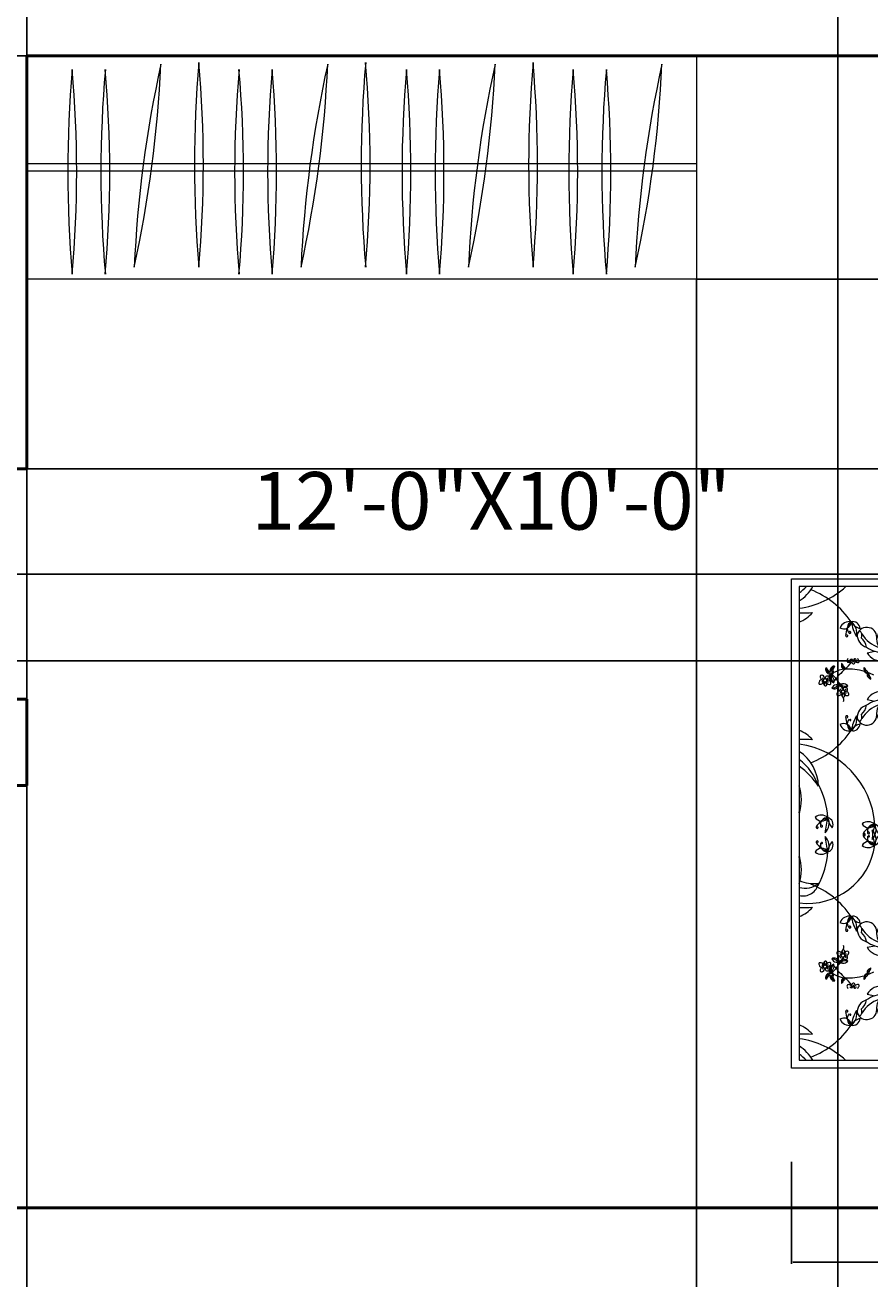
# Model space of a CAD drawing. Units: inches. Extents: x 3 to 576, y -689 to 51.
# Tile 5 of 21: x 111 to 199, y -514 to -383. Entities that reach past the tile are written whole.
import ezdxf

# ---------------------------------------------------------------- set-up
doc = ezdxf.new("R2010")
doc.units = ezdxf.units.IN
doc.header["$MEASUREMENT"] = 0
for name, color, linetype, lineweight in [('A-ANNO-DIMS', 2, 'Continuous', 18), ('A-AREA-IDEN', 7, 'Continuous', 18), ('A-FURN', 8, 'Continuous', 18), ('A-WALL', 7, 'Continuous', 50)]:
    doc.layers.add(name, color=color, linetype=linetype, lineweight=lineweight)
doc.styles.get("Standard").update_dxf_attribs({"font": 'arial.ttf'})
doc.dimstyles.get("Standard").update_dxf_attribs({"dimtxt": 0.18, "dimasz": 0.18, "dimexe": 0.18, "dimexo": 0.0625, "dimgap": 0.09, "dimtad": 0, "dimtih": 1, "dimtoh": 1, "dimdec": 0, "dimzin": 0, "dimdsep": 46, "dimlunit": 3, "dimtxsty": 'Standard', "dimcen": 0.09, "dimadec": 0, "dimazin": 0, "dimtfac": 1, "dimtdec": 0, "dimtofl": 0, "dimtmove": 0, "dimatfit": 3, "dimfxl": 1, "dimtolj": 1, "dimtzin": 0, "dimarcsym": 0})

# ---------------------------------------------------------------- blocks, each defined once
blk = doc.blocks.new('BED-DOUBLE')
for p, q in [((59.45, 69.91), (59.45, 0)), ((53.63, 58.35), (53.63, 67.49)), ((49.06, 62.92), (58.2, 62.92)), ((0, 60.68), (25.18, 60.68)), ((0, 9.72), (0, 60.68)), ((25.18, 60.68), (25.18, 56.73)), ((0.81, 59.87), (0.81, 10.53)), ((24.37, 59.87), (0.81, 59.87)), ((24.37, 56.73), (24.37, 59.87)), ((19.95, 13.6), (19.95, 56.73)), ((20.82, 13.66), (20.82, 56.73)), ((38.97, 55.99), (39.54, 56.55)), ((39.54, 56.55), (42.51, 54.01)), ((39.25, 53.16), (38.97, 55.99)), ((59.45, 55.93), (40.27, 55.93)), ((48.41, 55.93), (48.41, 13.98)), ((58.56, 13.98), (58.56, 55.93)), ((42.51, 54.01), (44.49, 51.31)), ((7.9, 52.98), (8.69, 53.14)), ((38.97, 49.62), (39.25, 53.16)), ((44.49, 51.31), (46.33, 46.22)), ((13.08, 20.76), (13.08, 49.15)), ((38.55, 46.5), (38.97, 49.62)), ((7.9, 48.1), (8.69, 47.94)), ((37.7, 44.66), (38.55, 46.5)), ((46.33, 46.22), (48.41, 38.59)), ((37.13, 42.39), (37.7, 44.66)), ((38.97, 42.11), (37.13, 42.39)), ((43.07, 40.55), (38.97, 42.11)), ((41.87, 14.23), (41.76, 41.05)), ((42.58, 14.23), (42.48, 40.78)), ((48.41, 36.72), (43.07, 40.55)), ((44.78, 14.2), (44.43, 39.58)), ((45.5, 14.17), (45.15, 39.06)), ((7.9, 22.3), (8.69, 22.46)), ((7.9, 17.41), (8.69, 17.26)), ((24.37, 10.53), (24.37, 13.61)), ((25.18, 13.59), (25.18, 9.72)), ((0.81, 10.53), (24.37, 10.53)), ((53.63, 11.56), (53.63, 2.42)), ((25.18, 9.72), (0, 9.72)), ((49.06, 6.99), (58.2, 6.99))]:
    blk.add_line(p, q)
for points in [[(47.8, 55.93), (47.8, 69.91), (59.45, 69.91)], [(53.63, 62.92), (52.22, 62.1)], [(53.63, 62.92), (55.04, 62.1)], [(59.45, 13.98), (47.8, 13.98), (47.8, 0), (59.45, 0)], [(53.63, 6.99), (52.22, 7.81)], [(53.63, 6.99), (55.04, 7.81)]]:
    blk.add_lwpolyline(points)
for points in [[(33.13, 56.7, 0.001242), (19.87, 56.73, -0.127202), (13.26, 58.14)], [(57.71, 51.91, 0.074897), (53.14, 51.83, -0.472817)], [(52.89, 35.28, 0.14099), (57.55, 35.14, 0.235245)], [(52.89, 32.3, -0.14099), (57.55, 32.44, -0.235245)], [(57.71, 18, -0.074897), (53.14, 18.08, 0.472817)], [(21.37, 13.68, 0.056112), (17.53, 13.18, 0.095341), (13.82, 12.19)]]:
    blk.add_lwpolyline(points, format="xyb")
for centre, radius in [((53.63, 62.92), 3.26), ((53.63, 62.92), 1.63), ((3.49, 50.11), 0.178), ((5.36, 48.94), 0.178), ((5.36, 21.45), 0.178), ((3.49, 20.29), 0.178), ((53.63, 6.99), 3.26), ((53.63, 6.99), 1.63)]:
    blk.add_circle(centre, radius)
for centre, radius, start, end in [((-2.47, 63.69), 5.54, 306.3036, 316.4814), ((-1.64, 62.09), 4.45, 303.4617, 330.1116), ((-0.42, 66.67), 9.13, 277.745, 311.8856), ((-1.32, 51.05), 9.13, 34.3865, 68.5908), ((13.3, 57.49), 0.645, 93.98, 207.3412), ((-0.61, 59.6), 3.71, 292.5547, 318.9546), ((1.38, 69.77), 12.63, 267.4081, 273.6519), ((6, 55.22), 1.01, 77.7115, 159.0387), ((5.45, 56.23), 0.762, 238.4633, 358.2869), ((7.95, 54.69), 2.31, 138.8402, 177.9352), ((6.56, 55.55), 0.747, 117.6827, 223.7762), ((6.39, 55.47), 0.757, 2.9516, 103.728), ((12.45, 57.59), 6.39, 192.5173, 207.1824), ((5.37, 55.04), 1.44, 345.4653, 54.2343), ((7.54, 57.02), 1.56, 211.3827, 255.2969), ((-59.69, 49.98), 72.78, 359.3433, 5.6887), ((37.8, 120.65), 64.12, 265.8294, 271.553), ((64.29, 55.36), 26.39, 177.4519, 191.3392), ((6.09, 55.1), 0.0988, 223.7762, 159.7183), ((7.84, 54.58), 1.05, 350.264, 160.8688), ((8.16, 54.83), 1.31, 175.969, 254.3045), ((6.7, 54.8), 0.643, 333.9755, 53.2681), ((10.15, 56.66), 3.3, 211.2614, 251.7045), ((10.53, 54.2), 1.67, 84.9449, 172.8857), ((11.17, 53.54), 1.62, 111.5819, 201.4221), ((10.7, 54.68), 1.18, 354.4856, 91.0538), ((8.16, 57.76), 5.29, 303.6671, 333.2997), ((5.76, 54.77), 0.113, 177.9352, 11.4834), ((5.81, 54.78), 0.0551, 11.4834, 127.9409), ((6.41, 53.42), 1.4, 6.1662, 51.5825), ((9.88, 56.69), 3.75, 236.2883, 266.5076), ((10.9, 54.49), 2.03, 182.3591, 234.0401), ((9.83, 55.04), 2.1, 265.2933, 346.921), ((6.09, 52.15), 0.294, 127.7621, 169.0403), ((5.94, 52.4), 0.414, 265.053, 338.3618), ((6.48, 51.84), 0.541, 113.4276, 137.6104), ((6.42, 52.4), 0.178, 183.2768, 356.7232), ((6.55, 52.07), 0.291, 139.7889, 227.6792), ((6.25, 52.01), 0.368, 350.3487, 43.6538), ((6.93, 52.39), 0.428, 198.7263, 262.5032), ((6.59, 52.19), 0.17, 1.1081, 91.8675), ((6.7, 52.15), 0.297, 11.5637, 52.6358), ((9.4, 53.85), 1.74, 209.9085, 343.1337), ((10.13, 52.75), 0.434, 167.3041, 285.1471), ((11.31, 50.67), 2.7, 122.7011, 126.3445), ((11.81, 53.58), 2.23, 199.2822, 299.1751), ((10.62, 50.95), 1.43, 41.5653, 105.1471), ((12.57, 55.82), 2.9, 238.8218, 279.1554), ((11.31, 50.67), 2.7, 55.785, 94.7304), ((12.31, 52.24), 0.842, 30.0293, 52.325), ((3.75, 51.26), 0.199, 124.3538, 214.3923), ((4.04, 51.23), 0.464, 190.3057, 287.1958), ((4.17, 51.39), 0.538, 176.9701, 248.2913), ((8.01, 54.23), 5.2, 212.6784, 216.3746), ((3.99, 51.27), 0.206, 216.3746, 291.7548), ((4.48, 51.12), 0.464, 122.8155, 187.3992), ((4.12, 50.93), 0.155, 289.3605, 111.7548), ((4.24, 50.93), 0.155, 221.8703, 44.2646), ((4.69, 51.06), 0.538, 109.4799, 177.6828), ((4.4, 51.4), 0.199, 56.8636, 146.9021), ((4.5, 51.18), 0.206, 148.8844, 224.2646), ((8.78, 48.6), 5.2, 145.1882, 148.8844), ((5.81, 48.38), 2.9, 94.756, 119.2041), ((11.99, 44.2), 9.55, 132.2412, 142.1744), ((7.17, 51.8), 1.97, 178.3264, 187.1302), ((5.04, 51.53), 0.367, 11.3256, 64.4621), ((6.29, 52.06), 1.1, 190.2588, 210.656), ((5.55, 51.61), 0.336, 188.3432, 274.2869), ((5.84, 51.79), 0.586, 210.656, 242.6341), ((6.28, 52.3), 1.12, 218.2101, 226.3071), ((5.45, 51.35), 0.142, 325.7657, 67.4417), ((1.03, 56.11), 6.64, 313.1541, 322.0459), ((5.96, 45.49), 5.79, 73.5842, 93.8277), ((5.91, 52.13), 0.137, 142.4737, 265.053), ((6.46, 51.97), 0.153, 227.6792, 350.3487), ((5.87, 52.08), 0.583, 353.0852, 15.7171), ((6.91, 52.1), 0.138, 255.2356, 54.9248), ((9.52, 51.39), 1.97, 178.3264, 187.1302), ((7.39, 51.11), 0.367, 11.3256, 64.4621), ((8.64, 51.64), 1.1, 190.2588, 210.656), ((7.9, 51.19), 0.336, 188.3432, 274.2869), ((8.19, 51.38), 0.586, 210.656, 242.6341), ((8.64, 51.88), 1.12, 218.2101, 226.3071), ((7.81, 50.93), 0.142, 325.7657, 67.4417), ((11.41, 53.92), 2.01, 277.436, 299.9149), ((12.48, 52.59), 1.05, 221.5653, 293.8354), ((12.31, 52.24), 0.842, 314.4517, 333.558), ((58.53, 49.42), 9.37, 165.1039, 191.0369), ((51.31, 43.01), 9.01, 65.1316, 101.7583), ((723.03, 13.38), 666.43, 176.68521, 177.14978), ((2.98, 49.84), 0.137, 142.4737, 265.053), ((3.16, 49.87), 0.294, 61.2196, 169.0403), ((3, 50.12), 0.414, 265.053, 338.3618), ((3.35, 50.47), 0.351, 157.4086, 261.4386), ((3.15, 50.48), 0.176, 58.0499, 135.6268), ((3.55, 49.55), 0.541, 113.4276, 137.6104), ((3.34, 50.37), 0.118, 172.906, 277.132), ((2.95, 50.16), 0.561, 14.7558, 58.0499), ((3.62, 49.79), 0.291, 139.7889, 227.6792), ((3.53, 49.68), 0.153, 227.6792, 350.3487), ((3.74, 50.31), 0.243, 36.1046, 181.4281), ((2.93, 49.79), 0.583, 353.0852, 15.7171), ((3.31, 49.72), 0.368, 350.3487, 43.6538), ((3.59, 50.5), 0.245, 270.0645, 331.1507), ((3.8, 50.44), 0.28, 221.8413, 265.7877), ((4, 50.1), 0.428, 198.7263, 262.5032), ((3.66, 49.9), 0.17, 1.1081, 91.8675), ((3.8, 50.33), 0.174, 263.7526, 41.7054), ((3.76, 49.86), 0.297, 11.5637, 86.365), ((5.81, 48.38), 2.9, 124.0033, 132.4917), ((3.98, 49.81), 0.138, 255.2356, 54.9248), ((2.83, 48.01), 3.1, 63.7819, 68.2913), ((4.48, 50.4), 0.493, 128.3208, 208.8162), ((4.57, 50.43), 0.59, 207.7043, 254.3516), ((4.94, 50.48), 0.812, 157.2305, 229.0635), ((4.67, 50.75), 0.478, 174.4544, 220.6188), ((4.19, 50.1), 0.812, 270.278, 342.111), ((4.73, 49.08), 0.574, 98.7227, 159.3375), ((1.96, 48.08), 3.48, 30.544, 49.818), ((3.87, 50.06), 0.574, 340.0041, 40.6188), ((4.57, 50.12), 0.478, 278.7227, 324.8872), ((4.49, 49.73), 0.493, 290.5253, 358.5375), ((5.45, 49.87), 0.493, 182.8499, 266.1226), ((5.26, 50.22), 0.478, 231.7607, 277.9252), ((5.63, 50.31), 0.812, 214.5369, 286.3699), ((5.4, 49.18), 0.574, 37.3105, 97.9252), ((8.21, 50.67), 0.336, 147.5332, 233.4768), ((7.94, 50.71), 0.142, 354.3784, 96.0543), ((8.51, 50.85), 0.586, 179.1859, 211.164), ((5.96, 45.49), 5.79, 63.0032, 69.8941), ((8.95, 51.12), 1.1, 211.164, 231.5612), ((9.15, 52.01), 1.97, 234.6898, 243.4936), ((9.16, 51), 1.12, 195.5129, 203.6099), ((7.9, 50.27), 0.367, 357.3579, 50.4944), ((9.48, 50.34), 0.135, 12.7051, 190.4384), ((9.56, 50.36), 0.219, 190.4384, 10.4136), ((11.81, 47.5), 2.23, 60.8249, 160.7178), ((32.84, 49.05), 5.69, 336.2616, 11.3392), ((4.44, 49.82), 0.59, 244.9899, 291.6373), ((4.85, 48.67), 0.137, 142.4737, 265.053), ((5.03, 48.7), 0.294, 61.2196, 169.0403), ((4.88, 48.95), 0.414, 265.053, 338.3618), ((5.23, 49.31), 0.351, 157.4086, 261.4386), ((5.03, 49.32), 0.176, 58.0499, 135.6268), ((5.43, 48.38), 0.541, 113.4276, 137.6104), ((5.21, 49.21), 0.118, 172.906, 277.132), ((4.83, 48.99), 0.561, 14.7558, 58.0499), ((1.96, 48.08), 3.48, 23.0501, 23.8477), ((5.5, 48.62), 0.291, 139.7889, 227.6792), ((5.4, 48.52), 0.153, 227.6792, 350.3487), ((5.61, 49.14), 0.243, 36.1046, 181.4281), ((4.81, 48.63), 0.583, 353.0852, 15.7171), ((5.47, 49.97), 0.59, 265.0106, 311.658), ((1.96, 48.08), 3.48, 357.1071, 4.7585), ((5.19, 48.56), 0.368, 350.3487, 43.6538), ((5.47, 49.33), 0.245, 270.0645, 331.1507), ((5.68, 49.27), 0.28, 221.8413, 265.7877), ((5.87, 48.94), 0.428, 198.7263, 262.5032), ((5.53, 48.74), 0.17, 1.1081, 91.8675), ((5.68, 49.17), 0.174, 263.7526, 41.7054), ((5.64, 48.7), 0.297, 11.5637, 86.365), ((5.85, 48.65), 0.138, 255.2356, 54.9248), ((9.4, 47.23), 1.74, 16.8663, 150.0915), ((10.13, 48.33), 0.434, 74.8529, 192.6959), ((10.62, 50.13), 1.43, 254.8529, 318.4347), ((11.41, 47.16), 2.01, 60.0851, 82.564), ((12.48, 48.49), 1.05, 66.1646, 138.4347), ((12.31, 48.84), 0.842, 307.675, 336.7144), ((12.31, 48.84), 0.842, 23.229, 45.5483), ((8.16, 46.25), 1.31, 105.6955, 184.031), ((6.41, 47.66), 1.4, 308.4175, 353.8338), ((10.15, 44.42), 3.3, 108.2955, 148.7386), ((9.88, 44.39), 3.75, 93.4924, 123.7117), ((10.9, 46.59), 2.03, 125.9599, 177.6409), ((11.17, 47.54), 1.62, 158.5779, 248.4181), ((9.83, 46.04), 2.1, 13.079, 94.7067), ((11.31, 50.41), 2.7, 233.6555, 237.2989), ((12.57, 45.26), 2.9, 79.7133, 121.1782), ((11.31, 50.41), 2.7, 265.2696, 304.215), ((8.16, 43.32), 5.29, 21.4941, 56.3329), ((65.19, 44.49), 16.25, 168.0397, 199.2615), ((5.76, 46.31), 0.113, 348.5166, 182.0648), ((7.95, 46.39), 2.31, 182.0648, 221.1598), ((5.81, 46.3), 0.0551, 232.0591, 348.5166), ((6.56, 45.54), 0.747, 136.2238, 242.3173), ((6.13, 45.97), 0.0595, 200.2667, 136.2271), ((5.37, 46.05), 1.44, 305.7657, 14.5347), ((12.45, 43.49), 6.39, 152.8176, 167.4827), ((7.84, 46.5), 1.05, 199.1312, 9.736), ((6.7, 46.28), 0.643, 306.7319, 26.0245), ((10.53, 46.88), 1.67, 187.1143, 275.0551), ((10.7, 46.4), 1.18, 268.9462, 5.5144), ((63.55, 37.54), 27.11, 160.1194, 169.3383), ((32.41, 42.33), 25.35, 352.2196, 9.497), ((-0.61, 41.48), 3.71, 41.0454, 67.4453), ((-1.32, 50.03), 9.13, 291.4092, 325.6135), ((5.45, 44.85), 0.762, 1.7131, 121.5367), ((6, 45.86), 1.01, 200.9613, 282.2885), ((6.39, 45.61), 0.757, 256.272, 357.0484), ((7.54, 44.06), 1.56, 104.7031, 148.6173), ((1.38, 31.32), 12.63, 86.3481, 92.5919), ((-0.42, 34.41), 9.13, 4.4623, 82.255), ((-1.64, 38.99), 4.45, 1.272, 56.5383), ((-2.47, 37.39), 5.54, 17.8504, 53.6964), ((37.07, 42.55), 0.169, 178.8623, 289.7536), ((-4.03, 34.48), 8.25, 34.0123, 54.053), ((-5.31, 35.11), 9.13, 4.4623, 27.4146), ((61.64, 37.91), 12.33, 169.8617, 193.6238), ((45.23, 36.98), 12.46, 351.5249, 13.96), ((-3.99, 37.66), 5.02, 343.5431, 17.0202), ((-6.58, 35.67), 7.42, 4.3787, 5.6357), ((-11.66, 31.77), 13.27, 19.7217, 19.9028), ((3.11, 35.07), 1.01, 47.7873, 129.1145), ((3.14, 36.22), 0.762, 208.5391, 328.3627), ((4.54, 33.64), 2.31, 108.9159, 148.011), ((3.76, 35.07), 0.747, 87.7585, 193.852), ((9.89, 33.91), 6.39, 162.593, 177.2582), ((2.48, 35.23), 1.44, 315.5411, 24.3101), ((5.35, 35.86), 1.56, 181.4585, 225.3727), ((3.58, 35.09), 0.757, 333.0274, 73.8037), ((8, 34.37), 1.01, 47.7873, 129.1145), ((50.55, 43.52), 8.57, 264.0129, 285.8293), ((2.68, 34.8), 0.113, 148.011, 341.5592), ((2.73, 34.78), 0.0551, 341.5592, 98.0167), ((3.13, 34.92), 0.0988, 193.852, 129.9245), ((8.03, 35.52), 0.762, 208.5391, 328.3627), ((7.57, 34.1), 0.113, 148.011, 341.5592), ((7.57, 33.97), 0.113, 18.4408, 211.989), ((9.43, 32.94), 2.31, 108.9159, 148.011), ((7.62, 34.08), 0.0551, 341.5592, 98.0167), ((7.62, 33.99), 0.0551, 261.9833, 18.4408), ((8.65, 34.38), 0.747, 87.7585, 193.852), ((8.02, 34.22), 0.0988, 193.852, 129.9245), ((7.37, 34.53), 1.44, 315.5411, 24.3101), ((14.78, 33.21), 6.39, 162.593, 177.2582), ((7.37, 33.54), 1.44, 335.6899, 44.4589), ((14.78, 34.86), 6.39, 182.7418, 197.407), ((8.47, 34.4), 0.757, 333.0274, 73.8037), ((10.24, 35.16), 1.56, 181.4585, 225.3727), ((8.47, 33.67), 0.757, 286.1963, 26.9726), ((10.24, 32.91), 1.56, 134.6273, 178.5415), ((1.69, 33.95), 7.07, 262.8636, 351.8197), ((2.68, 33.27), 0.113, 18.4408, 211.989), ((4.54, 34.43), 2.31, 211.989, 251.0841), ((2.73, 33.29), 0.0551, 261.9833, 18.4408), ((3.76, 32.99), 0.747, 166.148, 272.2415), ((3.17, 33.16), 0.0595, 230.1909, 166.0209), ((9.89, 34.16), 6.39, 182.7418, 197.407), ((2.48, 32.84), 1.44, 335.6899, 44.4589), ((5.35, 32.21), 1.56, 134.6273, 178.5415), ((3.58, 32.97), 0.757, 286.1963, 26.9726), ((8.03, 32.55), 0.762, 31.6373, 151.4609), ((8, 33.7), 1.01, 230.8855, 312.2127), ((9.43, 35.13), 2.31, 211.989, 251.0841), ((8.65, 33.69), 0.747, 166.148, 272.2415), ((8.06, 33.86), 0.0595, 230.1909, 166.0209), ((-3.99, 30.4), 5.02, 342.9798, 16.4569), ((-6.58, 32.39), 7.42, 354.3643, 355.6213), ((-11.66, 36.3), 13.27, 340.0972, 340.2783), ((3.14, 31.85), 0.762, 31.6373, 151.4609), ((3.11, 33), 1.01, 230.8855, 312.2127), ((-5.31, 32.96), 9.13, 332.5854, 355.5377), ((53.02, 31.01), 3.71, 155.0183, 198.5407), ((50.55, 24.06), 8.57, 74.1707, 95.9871), ((54.23, 31.48), 3.46, 333.3437, 16.1026), ((2.33, 33.04), 4.09, 248.117, 276.6195), ((1.2, 29.29), 1.64, 256.3898, 349.0739), ((1.42, 30.52), 2.07, 252.8609, 311.9049), ((-1.32, 20.37), 9.13, 34.3865, 68.5908), ((57.84, 24.53), 8.9, 153.8761, 196.1746), ((45.48, 26.29), 12.29, 346.3427, 11.1841), ((1.38, 39.08), 12.63, 267.4081, 273.6519), ((-0.61, 28.92), 3.71, 292.5547, 318.9546), ((6, 24.53), 1.01, 77.7115, 159.0387), ((5.45, 25.55), 0.762, 238.4633, 358.2869), ((7.95, 24), 2.31, 138.8402, 177.9352), ((6.56, 24.86), 0.747, 117.6827, 223.7762), ((6.39, 24.79), 0.757, 2.9516, 103.728), ((7.54, 26.34), 1.56, 211.3827, 255.2969), ((5.37, 24.35), 1.44, 345.4653, 54.2343), ((12.45, 26.91), 6.39, 192.5173, 207.1824), ((7.84, 23.9), 1.05, 350.264, 160.8688), ((10.53, 23.52), 1.67, 84.9449, 172.8857), ((10.7, 24), 1.18, 354.4856, 91.0538), ((8.16, 27.08), 5.29, 303.6671, 338.5059), ((5.76, 24.08), 0.113, 177.9352, 11.4834), ((5.81, 24.09), 0.0551, 11.4834, 127.9409), ((6.09, 24.41), 0.0988, 223.7762, 159.7183), ((8.16, 24.15), 1.31, 175.969, 254.3045), ((6.7, 24.12), 0.643, 333.9755, 53.2681), ((6.41, 22.74), 1.4, 6.1662, 51.5825), ((10.15, 25.98), 3.3, 211.2614, 251.7045), ((10.9, 23.81), 2.03, 182.3591, 234.0401), ((11.17, 22.86), 1.62, 111.5819, 201.4221), ((9.83, 24.36), 2.1, 265.2933, 346.921), ((1.96, 22.32), 3.48, 355.2415, 2.8929), ((9.88, 26.01), 3.75, 236.2883, 266.5076), ((9.4, 23.17), 1.74, 209.9085, 343.1337), ((11.31, 19.99), 2.7, 122.7011, 126.3445), ((12.57, 25.14), 2.9, 238.8218, 280.2867), ((11.31, 19.99), 2.7, 55.785, 94.7304), ((12.31, 21.55), 0.842, 23.2856, 52.325), ((58.53, 20.49), 9.37, 168.9631, 194.8961), ((723.03, 56.53), 666.43, 182.85022, 183.31479), ((4.44, 20.58), 0.59, 68.3627, 115.0101), ((4.19, 20.3), 0.812, 17.889, 89.722), ((4.73, 21.32), 0.574, 200.6625, 261.2773), ((4.49, 20.66), 0.493, 1.4625, 69.4747), ((4.85, 21.72), 0.137, 94.947, 217.5263), ((5.03, 21.7), 0.294, 190.9597, 298.7804), ((4.88, 21.45), 0.414, 21.6382, 94.947), ((5.23, 21.09), 0.351, 98.5614, 202.5914), ((5.03, 21.08), 0.176, 224.3732, 301.9501), ((5.45, 20.52), 0.493, 93.8774, 177.1501), ((5.63, 20.09), 0.812, 73.6301, 145.4631), ((5.43, 22.01), 0.541, 222.3896, 246.5724), ((5.21, 21.19), 0.118, 82.868, 187.094), ((4.83, 21.41), 0.561, 301.9501, 345.2442), ((1.96, 22.32), 3.48, 336.1523, 336.9499), ((5.5, 21.78), 0.291, 132.3208, 220.2111), ((5.4, 21.88), 0.153, 9.6513, 132.3208), ((4.81, 21.77), 0.583, 344.2829, 6.9148), ((5.61, 21.26), 0.243, 178.5719, 323.8954), ((5.47, 20.43), 0.59, 48.342, 94.9894), ((5.19, 21.84), 0.368, 316.3462, 9.6513), ((5.87, 21.46), 0.428, 97.4968, 161.2737), ((5.68, 21.12), 0.28, 94.2123, 138.1587), ((5.47, 21.07), 0.245, 28.8493, 89.9355), ((5.53, 21.66), 0.17, 268.1325, 358.8919), ((5.64, 21.7), 0.297, 273.635, 348.4363), ((5.68, 21.23), 0.174, 318.2946, 96.2474), ((5.85, 21.75), 0.138, 305.0752, 104.7644), ((10.13, 22.07), 0.434, 167.3041, 285.1471), ((11.81, 22.9), 2.23, 199.2822, 299.1751), ((10.62, 20.26), 1.43, 41.5653, 105.1471), ((11.41, 23.23), 2.01, 277.436, 299.9149), ((12.48, 21.91), 1.05, 221.5653, 293.8354), ((12.31, 21.55), 0.842, 314.4517, 336.7144), ((2.98, 20.56), 0.137, 94.947, 217.5263), ((3.16, 20.53), 0.294, 190.9597, 298.7804), ((3, 20.28), 0.414, 21.6382, 94.947), ((3.35, 19.93), 0.351, 98.5614, 202.5914), ((3.15, 19.91), 0.176, 224.3732, 301.9501), ((3.55, 20.85), 0.541, 222.3896, 246.5724), ((3.34, 20.03), 0.118, 82.868, 187.094), ((2.95, 20.24), 0.561, 301.9501, 345.2442), ((3.62, 20.61), 0.291, 132.3208, 220.2111), ((3.53, 20.71), 0.153, 9.6513, 132.3208), ((2.93, 20.61), 0.583, 344.2829, 6.9148), ((3.74, 20.09), 0.243, 178.5719, 323.8954), ((3.31, 20.68), 0.368, 316.3462, 9.6513), ((4.04, 19.17), 0.464, 72.8042, 169.6943), ((4, 20.3), 0.428, 97.4968, 161.2737), ((3.8, 19.96), 0.28, 94.2123, 138.1587), ((3.59, 19.9), 0.245, 28.8493, 89.9355), ((3.66, 20.5), 0.17, 268.1325, 358.8919), ((3.76, 20.54), 0.297, 273.635, 348.4363), ((3.8, 20.07), 0.174, 318.2946, 96.2474), ((5.81, 22.02), 2.9, 227.5083, 235.9967), ((3.98, 20.59), 0.138, 305.0752, 104.7644), ((2.83, 22.39), 3.1, 291.7087, 296.2181), ((4.48, 20), 0.493, 151.1838, 231.6792), ((4.57, 19.96), 0.59, 105.6484, 152.2957), ((4.12, 19.47), 0.155, 248.2452, 70.6395), ((4.94, 19.92), 0.812, 130.9365, 202.7695), ((4.24, 19.47), 0.155, 315.7354, 138.1297), ((4.67, 19.65), 0.478, 139.3812, 185.5456), ((1.96, 22.32), 3.48, 310.182, 329.456), ((3.87, 20.33), 0.574, 319.3812, 19.9959), ((11.99, 26.2), 9.55, 217.8256, 227.7588), ((4.57, 20.28), 0.478, 35.1128, 81.2773), ((5.26, 20.18), 0.478, 82.0748, 128.2393), ((5.4, 21.22), 0.574, 262.0748, 322.6895), ((8.21, 19.72), 0.336, 126.5232, 212.4668), ((8.51, 19.55), 0.586, 148.836, 180.8141), ((7.94, 19.68), 0.142, 263.9457, 5.6216), ((5.96, 24.9), 5.79, 290.1059, 296.9968), ((8.95, 19.28), 1.1, 128.4388, 148.836), ((9.15, 18.38), 1.97, 116.5064, 125.3102), ((9.16, 19.4), 1.12, 156.3901, 164.4871), ((7.9, 20.13), 0.367, 309.5056, 2.6421), ((9.56, 20.04), 0.219, 349.5864, 169.5616), ((9.48, 20.06), 0.135, 169.5616, 347.2949), ((-54.91, 18.62), 68.03, 355.2402, 1.8035), ((3.75, 19.14), 0.199, 145.6077, 235.6462), ((4.17, 19.01), 0.538, 111.7087, 183.0299), ((8.01, 16.17), 5.2, 143.6254, 147.3216), ((3.99, 19.13), 0.206, 68.2452, 143.6254), ((4.48, 19.27), 0.464, 172.6008, 237.1845), ((4.69, 19.33), 0.538, 182.3172, 250.5201), ((4.4, 18.99), 0.199, 213.0979, 303.1364), ((4.5, 19.21), 0.206, 135.7354, 211.1156), ((8.78, 21.8), 5.2, 211.1156, 214.8118), ((5.81, 22.02), 2.9, 240.7959, 265.244), ((6.29, 18.34), 1.1, 149.344, 169.7412), ((7.17, 18.6), 1.97, 172.8698, 181.6736), ((5.04, 18.87), 0.367, 295.5379, 348.6744), ((5.55, 18.79), 0.336, 85.7131, 171.6568), ((5.84, 18.61), 0.586, 117.3659, 149.344), ((6.28, 18.1), 1.12, 133.6929, 141.7899), ((5.45, 19.05), 0.142, 292.5583, 34.2343), ((5.96, 24.9), 5.79, 266.1723, 286.4158), ((1.03, 14.28), 6.64, 37.9541, 46.8459), ((5.91, 18.27), 0.137, 94.947, 217.5263), ((5.94, 18), 0.414, 21.6382, 94.947), ((6.55, 18.32), 0.291, 132.3208, 220.2111), ((6.46, 18.43), 0.153, 9.6513, 132.3208), ((5.87, 18.32), 0.583, 344.2829, 6.9148), ((6.25, 18.39), 0.368, 316.3462, 9.6513), ((6.93, 18.01), 0.428, 97.4968, 161.2737), ((6.91, 18.3), 0.138, 305.0752, 104.7644), ((8.64, 18.76), 1.1, 149.344, 169.7412), ((9.52, 19.01), 1.97, 172.8698, 181.6736), ((7.39, 19.29), 0.367, 295.5379, 348.6744), ((7.9, 19.21), 0.336, 85.7131, 171.6568), ((8.19, 19.02), 0.586, 117.3659, 149.344), ((8.64, 18.52), 1.12, 133.6929, 141.7899), ((7.81, 19.46), 0.142, 292.5583, 34.2343), ((9.4, 16.55), 1.74, 16.8663, 150.0915), ((11.81, 16.82), 2.23, 60.8249, 160.7178), ((10.62, 19.45), 1.43, 254.8529, 318.4347), ((11.41, 16.48), 2.01, 60.0851, 82.564), ((12.48, 17.81), 1.05, 66.1646, 138.4347), ((12.31, 18.16), 0.842, 16.6343, 45.5483), ((51.31, 26.9), 9.01, 258.2417, 294.8684), ((6.09, 18.24), 0.294, 190.9597, 232.2379), ((6.48, 18.56), 0.541, 222.3896, 246.5724), ((6.42, 18), 0.178, 3.2768, 176.7232), ((6.59, 18.21), 0.17, 268.1325, 358.8919), ((6.7, 18.25), 0.297, 307.3642, 348.4363), ((9.88, 13.7), 3.75, 93.4924, 123.7117), ((10.9, 15.91), 2.03, 125.9599, 177.6409), ((11.17, 16.86), 1.62, 158.5779, 248.4181), ((9.83, 15.35), 2.1, 13.079, 94.7067), ((10.13, 17.65), 0.434, 74.8529, 192.6959), ((11.31, 19.72), 2.7, 233.6555, 237.2989), ((12.57, 14.57), 2.9, 79.249, 121.1782), ((11.31, 19.72), 2.7, 265.2696, 304.215), ((8.16, 12.63), 5.29, 23.6453, 56.3329), ((12.31, 18.16), 0.842, 307.675, 342.5814), ((5.76, 15.63), 0.113, 348.5166, 182.0648), ((12.45, 12.81), 6.39, 152.8176, 167.4827), ((5.37, 15.36), 1.44, 305.7657, 14.5347), ((8.16, 15.56), 1.31, 105.6955, 184.031), ((7.84, 15.82), 1.05, 199.1312, 9.736), ((6.7, 15.6), 0.643, 306.7319, 26.0245), ((6.41, 16.98), 1.4, 308.4175, 353.8338), ((10.15, 13.74), 3.3, 108.2955, 148.7386), ((10.53, 16.2), 1.67, 187.1143, 275.0551), ((10.7, 15.72), 1.18, 268.9462, 5.5144), ((5.45, 14.17), 0.762, 1.7131, 121.5367), ((6, 15.18), 1.01, 200.9613, 282.2885), ((7.95, 15.71), 2.31, 182.0648, 221.1598), ((5.81, 15.62), 0.0551, 232.0591, 348.5166), ((6.56, 14.85), 0.747, 136.2238, 242.3173), ((6.13, 15.29), 0.0595, 200.2667, 136.2271), ((7.54, 13.38), 1.56, 104.7031, 148.6173), ((6.39, 14.93), 0.757, 256.272, 357.0484), ((-0.61, 10.8), 3.71, 41.0454, 67.4453), ((1.38, 0.63), 12.63, 86.3481, 92.5919), ((-1.32, 19.35), 9.13, 291.4092, 325.6135), ((35.29, -149.59), 163.86, 89.1145, 94.8735), ((39.86, -111.34), 125.62, 86.1, 90.9282), ((-0.42, 3.73), 9.13, 48.1144, 82.255), ((-1.64, 8.31), 4.45, 29.8884, 56.5383), ((13.47, 12.72), 0.637, 156.5219, 303.8264), ((-2.47, 6.71), 5.54, 43.5186, 53.6964)]:
    blk.add_arc(centre, radius, start, end)
blk = doc.blocks.new('*D18')
at = {"layer": 'A-ANNO-DIMS', "color": 0, "lineweight": -2, "transparency": 16777216}
for p, q in [((190.95, -501.53), (190.95, -512.13)), ((250.41, -501.53), (250.41, -512.13)), ((191.13, -511.95), (219.76, -511.95)), ((250.23, -511.95), (221.6, -511.95))]:
    blk.add_line(p, q, dxfattribs=at)
at = {"layer": 'A-ANNO-DIMS', "color": 0, "transparency": 16777216}
for points in [[(191.13, -511.92), (191.13, -511.98), (190.95, -511.95)], [(250.23, -511.92), (250.23, -511.98), (250.41, -511.95)]]:
    blk.add_solid(points, dxfattribs=at)
at = {"layer": 'Defpoints', "color": 0, "transparency": 16777216}
for p in [(190.95, -501.47), (250.41, -501.47), (250.41, -511.95)]:
    blk.add_point(p, dxfattribs=at)
at = {"layer": 'A-ANNO-DIMS', "color": 0, "transparency": 16777216, "insert": (220.68, -511.95), "char_height": 0.18, "attachment_point": 5}
blk.add_mtext('\\A1;4\'-11 1/2" TYP.', dxfattribs=at)
blk = doc.blocks.new('*D71')
at = {"layer": 'A-ANNO-DIMS', "color": 0, "lineweight": -2, "transparency": 16777216}
for p, q in [((531.23, -368.31), (2.66, -368.31)), ((2.84, -368.49), (2.84, -404.13)), ((2.84, -440.13), (2.84, -404.49)), ((531.23, -440.31), (2.66, -440.31))]:
    blk.add_line(p, q, dxfattribs=at)
at = {"layer": 'A-ANNO-DIMS', "color": 0, "transparency": 16777216}
for points in [[(2.81, -368.49), (2.87, -368.49), (2.84, -368.31)], [(2.81, -440.13), (2.87, -440.13), (2.84, -440.31)]]:
    blk.add_solid(points, dxfattribs=at)
at = {"layer": 'Defpoints', "color": 0, "transparency": 16777216}
for p in [(531.29, -368.31), (2.84, -440.31), (531.29, -440.31)]:
    blk.add_point(p, dxfattribs=at)
at = {"layer": 'A-ANNO-DIMS', "color": 0, "transparency": 16777216, "insert": (2.84, -404.31), "char_height": 0.18, "attachment_point": 5}
blk.add_mtext('\\A1;6\'-0"', dxfattribs=at)
blk = doc.blocks.new('*D72')
at = {"layer": 'A-ANNO-DIMS', "color": 0, "lineweight": -2, "transparency": 16777216}
for p, q in [((531.23, -440.31), (2.66, -440.31)), ((2.84, -440.49), (2.84, -444.63)), ((2.84, -449.13), (2.84, -444.99)), ((531.23, -449.31), (2.66, -449.31))]:
    blk.add_line(p, q, dxfattribs=at)
at = {"layer": 'A-ANNO-DIMS', "color": 0, "transparency": 16777216}
for points in [[(2.81, -440.49), (2.87, -440.49), (2.84, -440.31)], [(2.81, -449.13), (2.87, -449.13), (2.84, -449.31)]]:
    blk.add_solid(points, dxfattribs=at)
at = {"layer": 'Defpoints', "color": 0, "transparency": 16777216}
for p in [(531.29, -440.31), (2.84, -449.31), (531.29, -449.31)]:
    blk.add_point(p, dxfattribs=at)
at = {"layer": 'A-ANNO-DIMS', "color": 0, "transparency": 16777216, "insert": (2.84, -444.81), "char_height": 0.18, "attachment_point": 5}
blk.add_mtext('\\A1;0\'-9"', dxfattribs=at)
blk = doc.blocks.new('*D73')
at = {"layer": 'A-ANNO-DIMS', "color": 0, "lineweight": -2, "transparency": 16777216}
for p, q in [((531.23, -449.31), (2.66, -449.31)), ((2.84, -449.49), (2.84, -518.13)), ((2.84, -587.13), (2.84, -518.49)), ((531.23, -587.31), (2.66, -587.31))]:
    blk.add_line(p, q, dxfattribs=at)
at = {"layer": 'A-ANNO-DIMS', "color": 0, "transparency": 16777216}
for points in [[(2.81, -449.49), (2.87, -449.49), (2.84, -449.31)], [(2.81, -587.13), (2.87, -587.13), (2.84, -587.31)]]:
    blk.add_solid(points, dxfattribs=at)
at = {"layer": 'Defpoints', "color": 0, "transparency": 16777216}
for p in [(531.29, -449.31), (2.84, -587.31), (531.29, -587.31)]:
    blk.add_point(p, dxfattribs=at)
at = {"layer": 'A-ANNO-DIMS', "color": 0, "transparency": 16777216, "insert": (2.84, -518.31), "char_height": 0.18, "attachment_point": 5}
blk.add_mtext('\\A1;11\'-6"', dxfattribs=at)
blk = doc.blocks.new('*D86')
at = {"layer": 'A-ANNO-DIMS', "color": 0, "lineweight": -2, "transparency": 16777216}
for p, q in [((111.29, -97.21), (111.29, -688.94)), ((195.78, -97.21), (195.78, -688.94)), ((111.47, -688.76), (153, -688.76)), ((195.6, -688.76), (154.08, -688.76))]:
    blk.add_line(p, q, dxfattribs=at)
at = {"layer": 'A-ANNO-DIMS', "color": 0, "transparency": 16777216}
for points in [[(111.47, -688.73), (111.47, -688.79), (111.29, -688.76)], [(195.6, -688.73), (195.6, -688.79), (195.78, -688.76)]]:
    blk.add_solid(points, dxfattribs=at)
at = {"layer": 'Defpoints', "color": 0, "transparency": 16777216}
for p in [(111.29, -97.15), (195.78, -97.15), (195.78, -688.76)]:
    blk.add_point(p, dxfattribs=at)
at = {"layer": 'A-ANNO-DIMS', "color": 0, "transparency": 16777216, "insert": (153.54, -688.76), "char_height": 0.18, "attachment_point": 5}
blk.add_mtext('\\A1;7\'-0 1/2"', dxfattribs=at)
blk = doc.blocks.new('*D90')
at = {"layer": 'A-ANNO-DIMS', "color": 0, "lineweight": -2, "transparency": 16777216}
for p, q in [((111.29, -409.62), (111.29, -688.94)), ((181.04, -409.62), (181.04, -688.94)), ((111.47, -688.76), (145.63, -688.76)), ((180.86, -688.76), (146.7, -688.76))]:
    blk.add_line(p, q, dxfattribs=at)
at = {"layer": 'A-ANNO-DIMS', "color": 0, "transparency": 16777216}
for points in [[(111.47, -688.73), (111.47, -688.79), (111.29, -688.76)], [(180.86, -688.73), (180.86, -688.79), (181.04, -688.76)]]:
    blk.add_solid(points, dxfattribs=at)
at = {"layer": 'Defpoints', "color": 0, "transparency": 16777216}
for p in [(111.29, -409.56), (181.04, -409.56), (181.04, -688.76)]:
    blk.add_point(p, dxfattribs=at)
at = {"layer": 'A-ANNO-DIMS', "color": 0, "transparency": 16777216, "insert": (146.17, -688.76), "char_height": 0.18, "attachment_point": 5}
blk.add_mtext('\\A1;5\'-9 1/2"', dxfattribs=at)
blk = doc.blocks.new('*D91')
at = {"layer": 'A-ANNO-DIMS', "color": 0, "lineweight": -2, "transparency": 16777216}
for p, q in [((181.1, -386.31), (575.92, -386.31)), ((575.74, -386.49), (575.74, -397.75)), ((575.74, -409.38), (575.74, -398.11)), ((181.1, -409.56), (575.92, -409.56))]:
    blk.add_line(p, q, dxfattribs=at)
at = {"layer": 'A-ANNO-DIMS', "color": 0, "transparency": 16777216}
for points in [[(575.71, -386.49), (575.77, -386.49), (575.74, -386.31)], [(575.71, -409.38), (575.77, -409.38), (575.74, -409.56)]]:
    blk.add_solid(points, dxfattribs=at)
at = {"layer": 'Defpoints', "color": 0, "transparency": 16777216}
for p in [(181.04, -386.31), (181.04, -409.56), (575.74, -409.56)]:
    blk.add_point(p, dxfattribs=at)
at = {"layer": 'A-ANNO-DIMS', "color": 0, "transparency": 16777216, "insert": (575.74, -397.93), "char_height": 0.18, "attachment_point": 5}
blk.add_mtext('\\A1;1\'-11"', dxfattribs=at)
blk = doc.blocks.new('*D106')
at = {"layer": 'A-ANNO-DIMS', "color": 0, "lineweight": -2, "transparency": 16777216}
for p, q in [((111.36, -386.31), (575.92, -386.31)), ((575.74, -386.49), (575.74, -407.63)), ((575.74, -429.13), (575.74, -407.99)), ((111.36, -429.31), (575.92, -429.31))]:
    blk.add_line(p, q, dxfattribs=at)
at = {"layer": 'A-ANNO-DIMS', "color": 0, "transparency": 16777216}
for points in [[(575.71, -386.49), (575.77, -386.49), (575.74, -386.31)], [(575.71, -429.13), (575.77, -429.13), (575.74, -429.31)]]:
    blk.add_solid(points, dxfattribs=at)
at = {"layer": 'Defpoints', "color": 0, "transparency": 16777216}
for p in [(111.29, -386.31), (111.29, -429.31), (575.74, -429.31)]:
    blk.add_point(p, dxfattribs=at)
at = {"layer": 'A-ANNO-DIMS', "color": 0, "transparency": 16777216, "insert": (575.74, -407.81), "char_height": 0.18, "attachment_point": 5}
blk.add_mtext('\\A1;3\'-7"', dxfattribs=at)
blk = doc.blocks.new('*D125')
at = {"layer": 'A-ANNO-DIMS', "color": 0, "lineweight": -2, "transparency": 16777216}
for p, q in [((531.23, -368.31), (2.66, -368.31)), ((2.84, -368.49), (2.84, -377.13)), ((2.84, -386.13), (2.84, -377.49)), ((512.45, -386.31), (2.66, -386.31))]:
    blk.add_line(p, q, dxfattribs=at)
at = {"layer": 'A-ANNO-DIMS', "color": 0, "transparency": 16777216}
for points in [[(2.81, -368.49), (2.87, -368.49), (2.84, -368.31)], [(2.81, -386.13), (2.87, -386.13), (2.84, -386.31)]]:
    blk.add_solid(points, dxfattribs=at)
at = {"layer": 'Defpoints', "color": 0, "transparency": 16777216}
for p in [(531.29, -368.31), (2.84, -386.31), (512.51, -386.31)]:
    blk.add_point(p, dxfattribs=at)
at = {"layer": 'A-ANNO-DIMS', "color": 0, "transparency": 16777216, "insert": (2.84, -377.31), "char_height": 0.18, "attachment_point": 5}
blk.add_mtext('\\A1;1\'-6"', dxfattribs=at)

msp = doc.modelspace()

# ---------------------------------------------------------------- linework, layer by layer
at = {"layer": 'A-FURN'}
for p, q in [((181.04, -386.31), (111.29, -386.31)), ((111.29, -386.31), (111.29, -409.56)), ((181.04, -386.31), (181.04, -409.56)), ((181.04, -397.55), (111.29, -397.55)), ((181.04, -398.32), (111.29, -398.32)), ((181.04, -409.56), (111.29, -409.56))]:
    msp.add_line(p, q, dxfattribs=at)
for centre, start, end in [((237.88, -398.4), 175.0028, 184.9972), ((-5.83, -398.4), 355.0028, 4.9972), ((241.33, -398.4), 175.0028, 184.9972), ((-2.39, -398.4), 355.0028, 4.9972), ((3.05, -381.85), 347.508, 357.5023), ((244.69, -413.64), 167.508, 177.5023), ((251.07, -397.65), 175.0028, 184.9972), ((7.36, -397.65), 355.0028, 4.9972), ((255.26, -398.4), 175.0028, 184.9972), ((11.54, -398.4), 355.0028, 4.9972), ((258.7, -398.4), 175.0028, 184.9972), ((14.99, -398.4), 355.0028, 4.9972), ((20.43, -381.85), 347.508, 357.5023), ((262.06, -413.64), 167.508, 177.5023), ((268.45, -397.65), 175.0028, 184.9972), ((24.73, -397.65), 355.0028, 4.9972), ((272.7, -398.4), 175.0028, 184.9972), ((28.98, -398.4), 355.0028, 4.9972), ((276.14, -398.4), 175.0028, 184.9972), ((32.43, -398.4), 355.0028, 4.9972), ((279.5, -413.64), 167.508, 177.5023), ((37.87, -381.85), 347.508, 357.5023), ((285.89, -397.65), 175.0028, 184.9972), ((42.17, -397.65), 355.0028, 4.9972), ((290.07, -398.4), 175.0028, 184.9972), ((46.36, -398.4), 355.0028, 4.9972), ((293.52, -398.4), 175.0028, 184.9972), ((49.81, -398.4), 355.0028, 4.9972), ((296.88, -413.64), 167.508, 177.5023), ((55.25, -381.85), 347.508, 357.5023)]:
    msp.add_arc(centre, 122.32, start, end, dxfattribs=at)
at = {"layer": 'A-WALL'}
for p, q in [((111.29, -386.31), (111.29, -429.31)), ((111.29, -386.31), (219.29, -386.31)), ((102.29, -429.31), (111.29, -429.31)), ((47.29, -453.31), (111.29, -453.31)), ((111.29, -453.31), (111.29, -462.31)), ((47.29, -462.31), (111.29, -462.31)), ((47.29, -506.31), (255.29, -506.31))]:
    msp.add_line(p, q, dxfattribs=at)

# ---------------------------------------------------------------- block references
at = {"layer": 'A-FURN'}
msp.add_blockref('BED-DOUBLE', (190.95, -501.47), dxfattribs=at)

# ---------------------------------------------------------------- texts
at = {"layer": 'A-AREA-IDEN', "insert": (134.7, -429.66), "char_height": 6, "attachment_point": 1}
msp.add_mtext_dynamic_manual_height_columns('12\'-0"X10\'-0"', width=1.0156, gutter_width=1, heights=[0], dxfattribs=at)

# ---------------------------------------------------------------- dimensions: what is measured, and where the dimension line sits
at = {"layer": 'A-ANNO-DIMS'}
for base, p1, p2, picture, middle in [((195.78, -688.76), (111.29, -97.15), (195.78, -97.15), '*D86', (153.54, -688.76)), ((181.036, -688.7597), (111.294, -409.5571), (181.036, -409.5571), '*D90', (146.165, -688.7597))]:
    dim = msp.add_linear_dim(base=base, p1=p1, p2=p2, dimstyle='Standard', override={"dimdec": 1, "dimlfac": 1, "dimrnd": 0, "dimzin": 1, "dimdsep": 46, "dimlunit": 4, "dimfrac": 2}, dxfattribs=at)
    dim.commit()
    dim.dimension.update_dxf_attribs({"geometry": picture, "text_midpoint": middle})
for base, p1, p2, picture, middle in [((2.84, -440.31), (531.29, -368.31), (531.29, -440.31), '*D71', (2.84, -404.31)), ((2.84, -386.31), (531.29, -368.31), (512.51, -386.31), '*D125', (2.84, -377.31)), ((575.74, -429.31), (111.29, -386.31), (111.29, -429.31), '*D106', (575.74, -407.81)), ((575.744, -409.5571), (181.036, -386.3097), (181.036, -409.5571), '*D91', (575.744, -397.9334)), ((2.84, -449.31), (531.29, -440.31), (531.29, -449.31), '*D72', (2.84, -444.81)), ((2.84, -587.31), (531.29, -449.31), (531.29, -587.31), '*D73', (2.84, -518.31))]:
    dim = msp.add_linear_dim(base=base, p1=p1, p2=p2, angle=90, dimstyle='Standard', override={"dimdec": 1, "dimlfac": 1, "dimrnd": 0, "dimzin": 1, "dimdsep": 46, "dimlunit": 4, "dimfrac": 2}, dxfattribs=at)
    dim.commit()
    dim.dimension.update_dxf_attribs({"geometry": picture, "text_midpoint": middle})
dim = msp.add_linear_dim(base=(250.41, -511.95), p1=(190.95, -501.47), p2=(250.41, -501.47), text='<> TYP.', dimstyle='Standard', override={"dimdec": 1, "dimlfac": 1, "dimrnd": 0, "dimzin": 1, "dimdsep": 46, "dimlunit": 4, "dimfrac": 2}, dxfattribs=at)
dim.commit()
dim.dimension.update_dxf_attribs({"geometry": '*D18', "text_midpoint": (220.68, -511.95)})

doc.saveas('drawing.dxf')
